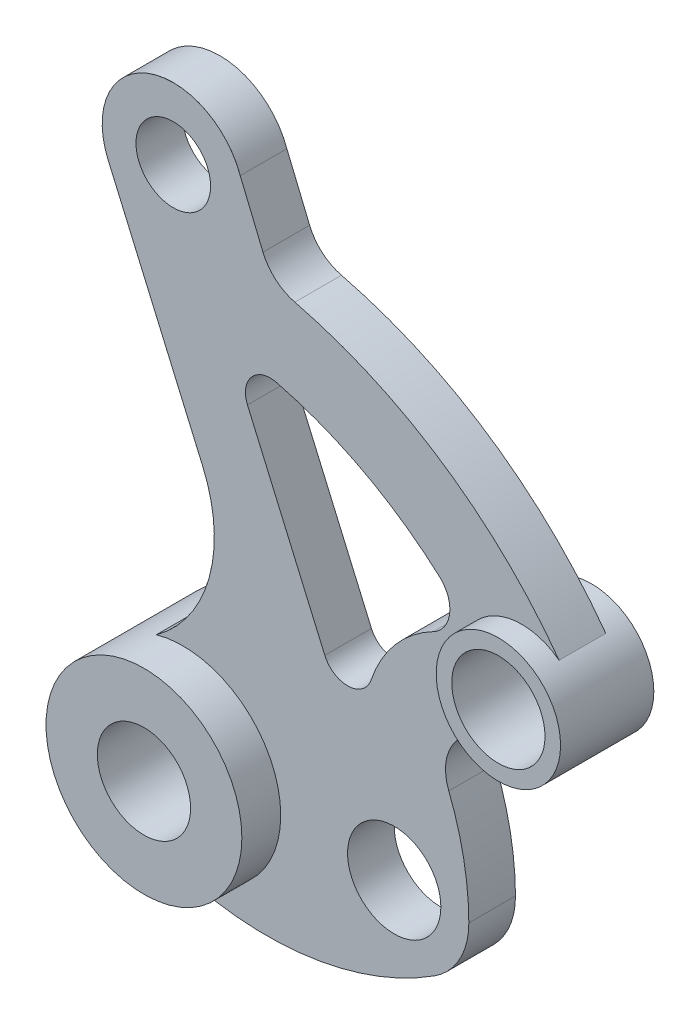
ISO-10303-21;
HEADER;
FILE_DESCRIPTION(('STEP AP214'),'2;1');
FILE_NAME('part.step','',(''),(''),'','','');
FILE_SCHEMA(('AUTOMOTIVE_DESIGN { 1 0 10303 214 1 1 1 1 }'));
ENDSEC;
DATA;
#1=APPLICATION_CONTEXT('core data for automotive mechanical design processes');
#2=APPLICATION_PROTOCOL_DEFINITION('international standard','automotive_design',2000,#1);
#3=PRODUCT_CONTEXT('',#1,'mechanical');
#4=PRODUCT('Part','Part','',(#3));
#5=PRODUCT_RELATED_PRODUCT_CATEGORY('part','',(#4));
#6=PRODUCT_DEFINITION_FORMATION('','',#4);
#7=PRODUCT_DEFINITION_CONTEXT('part definition',#1,'design');
#8=PRODUCT_DEFINITION('design','',#6,#7);
#9=PRODUCT_DEFINITION_SHAPE('','',#8);
#10=(LENGTH_UNIT() NAMED_UNIT(*) SI_UNIT(.MILLI.,.METRE.));
#11=(NAMED_UNIT(*) PLANE_ANGLE_UNIT() SI_UNIT($,.RADIAN.));
#12=(NAMED_UNIT(*) SI_UNIT($,.STERADIAN.) SOLID_ANGLE_UNIT());
#13=UNCERTAINTY_MEASURE_WITH_UNIT(LENGTH_MEASURE(1.E-05),#10,'distance_accuracy_value','');
#14=(GEOMETRIC_REPRESENTATION_CONTEXT(3) GLOBAL_UNCERTAINTY_ASSIGNED_CONTEXT((#13)) GLOBAL_UNIT_ASSIGNED_CONTEXT((#10,
#11,#12)) REPRESENTATION_CONTEXT('',''));
#15=CARTESIAN_POINT('',(0.,0.,0.));
#16=DIRECTION('',(0.,0.,1.));
#17=DIRECTION('',(1.,0.,0.));
#18=AXIS2_PLACEMENT_3D('',#15,#16,#17);
#19=CARTESIAN_POINT('',(0.,0.,15.));
#20=DIRECTION('',(0.,0.,1.));
#21=DIRECTION('',(1.,0.,0.));
#22=AXIS2_PLACEMENT_3D('',#19,#20,#21);
#23=PLANE('',#22);
#24=CARTESIAN_POINT('',(-3.06784573961168,163.971303350671,15.));
#25=DIRECTION('',(0.,0.,1.));
#26=DIRECTION('',(1.,0.,0.));
#27=AXIS2_PLACEMENT_3D('',#24,#25,#26);
#28=CIRCLE('',#27,12.000000000031);
#29=CARTESIAN_POINT('',(8.93215426041928,163.971303350671,15.));
#30=VERTEX_POINT('',#29);
#31=EDGE_CURVE('E225',#30,#30,#28,.T.);
#32=ORIENTED_EDGE('',*,*,#31,.F.);
#33=EDGE_LOOP('',(#32));
#34=FACE_BOUND('',#33,.T.);
#35=CARTESIAN_POINT('',(67.9996451646292,0.219675862409967,15.));
#36=DIRECTION('',(0.,0.,1.));
#37=DIRECTION('',(1.,0.,0.));
#38=AXIS2_PLACEMENT_3D('',#35,#36,#37);
#39=CIRCLE('',#38,14.9999999999901);
#40=CARTESIAN_POINT('',(82.9996451646192,0.219675862409967,15.));
#41=VERTEX_POINT('',#40);
#42=EDGE_CURVE('E222',#41,#41,#39,.T.);
#43=ORIENTED_EDGE('',*,*,#42,.F.);
#44=EDGE_LOOP('',(#43));
#45=FACE_BOUND('',#44,.T.);
#46=DIRECTION('',(0.398118875645799,-0.917333832829971,0.));
#47=VECTOR('',#46,1.);
#48=CARTESIAN_POINT('',(57.3020213071531,24.8688268965916,15.));
#49=LINE('',#48,#47);
#50=CARTESIAN_POINT('',(20.8018674677098,108.971410493279,15.));
#51=VERTEX_POINT('',#50);
#52=CARTESIAN_POINT('',(45.6745977520915,51.6603951145019,15.));
#53=VERTEX_POINT('',#52);
#54=EDGE_CURVE('E460',#51,#53,#49,.T.);
#55=ORIENTED_EDGE('',*,*,#54,.F.);
#56=CARTESIAN_POINT('',(28.1405381303495,112.156361498446,15.));
#57=DIRECTION('',(0.,0.,1.));
#58=DIRECTION('',(1.,0.,0.));
#59=AXIS2_PLACEMENT_3D('',#56,#57,#58);
#60=CIRCLE('',#59,7.99999999999999);
#61=CARTESIAN_POINT('',(30.0874281839262,119.915847249401,15.));
#62=VERTEX_POINT('',#61);
#63=EDGE_CURVE('E453',#51,#62,#60,.F.);
#64=ORIENTED_EDGE('',*,*,#63,.T.);
#65=CARTESIAN_POINT('',(0.,0.,15.));
#66=DIRECTION('',(0.,0.,1.));
#67=DIRECTION('',(1.,0.,0.));
#68=AXIS2_PLACEMENT_3D('',#65,#66,#67);
#69=CIRCLE('',#68,123.632777839312);
#70=CARTESIAN_POINT('',(82.5809627863903,92.0078710846932,15.));
#71=VERTEX_POINT('',#70);
#72=EDGE_CURVE('E455',#71,#62,#69,.T.);
#73=ORIENTED_EDGE('',*,*,#72,.F.);
#74=CARTESIAN_POINT('',(75.9014264830224,84.565842142799,15.));
#75=DIRECTION('',(0.,0.,1.));
#76=DIRECTION('',(1.,0.,0.));
#77=AXIS2_PLACEMENT_3D('',#74,#75,#76);
#78=CIRCLE('',#77,10.);
#79=CARTESIAN_POINT('',(80.5286057442506,75.7007864698515,15.));
#80=VERTEX_POINT('',#79);
#81=EDGE_CURVE('E446',#80,#71,#78,.T.);
#82=ORIENTED_EDGE('',*,*,#81,.F.);
#83=CARTESIAN_POINT('',(99.5000407152862,39.3540582107665,15.));
#84=DIRECTION('',(0.,0.,1.));
#85=DIRECTION('',(1.,0.,0.));
#86=AXIS2_PLACEMENT_3D('',#83,#84,#85);
#87=CIRCLE('',#86,41.);
#88=CARTESIAN_POINT('',(60.6029455250266,52.316156256989,15.));
#89=VERTEX_POINT('',#88);
#90=EDGE_CURVE('E447',#89,#80,#87,.F.);
#91=ORIENTED_EDGE('',*,*,#90,.F.);
#92=CARTESIAN_POINT('',(53.013268414732,54.8453461196665,15.));
#93=DIRECTION('',(0.,0.,1.));
#94=DIRECTION('',(1.,0.,0.));
#95=AXIS2_PLACEMENT_3D('',#92,#93,#94);
#96=CIRCLE('',#95,7.99999999999999);
#97=EDGE_CURVE('E394',#53,#89,#96,.T.);
#98=ORIENTED_EDGE('',*,*,#97,.F.);
#99=EDGE_LOOP('',(#55,#64,#73,#82,#91,#98));
#100=FACE_BOUND('',#99,.T.);
#101=DIRECTION('',(0.383451553640761,-0.923560992035982,0.));
#102=VECTOR('',#101,1.);
#103=CARTESIAN_POINT('',(76.5503269943444,31.7827864870954,15.));
#104=LINE('',#103,#102);
#105=CARTESIAN_POINT('',(18.3868968232772,171.872127002147,15.));
#106=VERTEX_POINT('',#105);
#107=CARTESIAN_POINT('',(25.7921859401268,154.036141991435,15.));
#108=VERTEX_POINT('',#107);
#109=EDGE_CURVE('E403',#106,#108,#104,.T.);
#110=ORIENTED_EDGE('',*,*,#109,.F.);
#111=CARTESIAN_POINT('',(-3.06784573961168,163.971303350671,15.));
#112=DIRECTION('',(0.,0.,1.));
#113=DIRECTION('',(1.,0.,0.));
#114=AXIS2_PLACEMENT_3D('',#111,#112,#113);
#115=CIRCLE('',#114,22.8632673258124);
#116=CARTESIAN_POINT('',(-24.0410943866144,154.869005069327,15.));
#117=VERTEX_POINT('',#116);
#118=EDGE_CURVE('E230',#106,#117,#115,.T.);
#119=ORIENTED_EDGE('',*,*,#118,.T.);
#120=DIRECTION('',(0.398118875645899,-0.917333832829927,0.));
#121=VECTOR('',#120,1.);
#122=CARTESIAN_POINT('',(6.41253141271611,84.6986539832474,15.));
#123=LINE('',#122,#121);
#124=CARTESIAN_POINT('',(6.4125314127161,84.6986539832473,15.));
#125=VERTEX_POINT('',#124);
#126=EDGE_CURVE('E214',#117,#125,#123,.T.);
#127=ORIENTED_EDGE('',*,*,#126,.T.);
#128=CARTESIAN_POINT('',(-34.876664402959,66.7793233904254,15.));
#129=DIRECTION('',(0.,0.,1.));
#130=DIRECTION('',(1.,0.,0.));
#131=AXIS2_PLACEMENT_3D('',#128,#129,#130);
#132=CIRCLE('',#131,45.0100000000001);
#133=CARTESIAN_POINT('',(-8.446752371103,30.346373331607,15.));
#134=VERTEX_POINT('',#133);
#135=EDGE_CURVE('E208',#125,#134,#132,.F.);
#136=ORIENTED_EDGE('',*,*,#135,.T.);
#137=CARTESIAN_POINT('',(0.,0.,15.));
#138=DIRECTION('',(0.,0.,1.));
#139=DIRECTION('',(1.,0.,0.));
#140=AXIS2_PLACEMENT_3D('',#137,#138,#139);
#141=CIRCLE('',#140,31.5);
#142=CARTESIAN_POINT('',(-2.21180302605378,-31.4222521053781,15.));
#143=VERTEX_POINT('',#142);
#144=EDGE_CURVE('E442',#134,#143,#141,.F.);
#145=ORIENTED_EDGE('',*,*,#144,.T.);
#146=CARTESIAN_POINT('',(27.0041064706894,64.2147210393117,15.));
#147=DIRECTION('',(0.,0.,1.));
#148=DIRECTION('',(1.,0.,0.));
#149=AXIS2_PLACEMENT_3D('',#146,#147,#148);
#150=CIRCLE('',#149,100.);
#151=CARTESIAN_POINT('',(80.9456047521891,-19.9892857724011,15.));
#152=VERTEX_POINT('',#151);
#153=EDGE_CURVE('E470',#143,#152,#150,.T.);
#154=ORIENTED_EDGE('',*,*,#153,.T.);
#155=CARTESIAN_POINT('',(67.9996451646292,0.219675862409967,15.));
#156=DIRECTION('',(0.,0.,1.));
#157=DIRECTION('',(1.,0.,0.));
#158=AXIS2_PLACEMENT_3D('',#155,#156,#157);
#159=CIRCLE('',#158,24.);
#160=CARTESIAN_POINT('',(91.999519928616,0.29720851973114,15.));
#161=VERTEX_POINT('',#160);
#162=EDGE_CURVE('E465',#152,#161,#159,.T.);
#163=ORIENTED_EDGE('',*,*,#162,.T.);
#164=CARTESIAN_POINT('',(0.,0.,15.));
#165=DIRECTION('',(0.,0.,1.));
#166=DIRECTION('',(1.,0.,0.));
#167=AXIS2_PLACEMENT_3D('',#164,#165,#166);
#168=CIRCLE('',#167,92.);
#169=CARTESIAN_POINT('',(85.5514368766947,33.8371341625282,15.));
#170=VERTEX_POINT('',#169);
#171=EDGE_CURVE('E464',#161,#170,#168,.T.);
#172=ORIENTED_EDGE('',*,*,#171,.T.);
#173=CARTESIAN_POINT('',(99.5000407152862,39.3540582107665,15.));
#174=DIRECTION('',(0.,0.,1.));
#175=DIRECTION('',(1.,0.,0.));
#176=AXIS2_PLACEMENT_3D('',#173,#174,#175);
#177=CIRCLE('',#176,15.);
#178=CARTESIAN_POINT('',(99.5862507147772,54.3538104699202,15.));
#179=VERTEX_POINT('',#178);
#180=EDGE_CURVE('E200',#170,#179,#177,.F.);
#181=ORIENTED_EDGE('',*,*,#180,.T.);
#182=CARTESIAN_POINT('',(108.999645164629,72.,15.));
#183=DIRECTION('',(0.,0.,1.));
#184=DIRECTION('',(1.,0.,0.));
#185=AXIS2_PLACEMENT_3D('',#182,#183,#184);
#186=CIRCLE('',#185,20.);
#187=CARTESIAN_POINT('',(121.045727624012,87.9653342395873,15.));
#188=VERTEX_POINT('',#187);
#189=EDGE_CURVE('E203',#179,#188,#186,.F.);
#190=ORIENTED_EDGE('',*,*,#189,.T.);
#191=CARTESIAN_POINT('',(0.,0.,15.));
#192=DIRECTION('',(0.,0.,1.));
#193=DIRECTION('',(1.,0.,0.));
#194=AXIS2_PLACEMENT_3D('',#191,#192,#193);
#195=CIRCLE('',#194,149.632777839312);
#196=CARTESIAN_POINT('',(36.0334160533632,145.229339774834,15.));
#197=VERTEX_POINT('',#196);
#198=EDGE_CURVE('E184',#188,#197,#195,.T.);
#199=ORIENTED_EDGE('',*,*,#198,.T.);
#200=CARTESIAN_POINT('',(39.6456008206666,159.787915296047,15.));
#201=DIRECTION('',(0.,0.,1.));
#202=DIRECTION('',(1.,0.,0.));
#203=AXIS2_PLACEMENT_3D('',#200,#201,#202);
#204=CIRCLE('',#203,15.);
#205=EDGE_CURVE('E197',#108,#197,#204,.T.);
#206=ORIENTED_EDGE('',*,*,#205,.F.);
#207=EDGE_LOOP('',(#110,#119,#127,#136,#145,#154,#163,#172,#181,#190,#199,#206));
#208=FACE_BOUND('',#207,.T.);
#209=ADVANCED_FACE('F50',(#34,#45,#100,#208),#23,.T.);
#210=CARTESIAN_POINT('',(0.,0.,0.));
#211=DIRECTION('',(0.,0.,1.));
#212=DIRECTION('',(1.,0.,0.));
#213=AXIS2_PLACEMENT_3D('',#210,#211,#212);
#214=PLANE('',#213);
#215=CARTESIAN_POINT('',(-3.06784573961168,163.971303350671,0.));
#216=DIRECTION('',(0.,0.,1.));
#217=DIRECTION('',(1.,0.,0.));
#218=AXIS2_PLACEMENT_3D('',#215,#216,#217);
#219=CIRCLE('',#218,12.000000000031);
#220=CARTESIAN_POINT('',(8.93215426041928,163.971303350671,0.));
#221=VERTEX_POINT('',#220);
#222=EDGE_CURVE('E221',#221,#221,#219,.T.);
#223=ORIENTED_EDGE('',*,*,#222,.T.);
#224=EDGE_LOOP('',(#223));
#225=FACE_BOUND('',#224,.T.);
#226=CARTESIAN_POINT('',(67.9996451646292,0.219675862409967,0.));
#227=DIRECTION('',(0.,0.,1.));
#228=DIRECTION('',(1.,0.,0.));
#229=AXIS2_PLACEMENT_3D('',#226,#227,#228);
#230=CIRCLE('',#229,14.9999999999901);
#231=CARTESIAN_POINT('',(82.9996451646192,0.219675862409967,0.));
#232=VERTEX_POINT('',#231);
#233=EDGE_CURVE('E218',#232,#232,#230,.T.);
#234=ORIENTED_EDGE('',*,*,#233,.T.);
#235=EDGE_LOOP('',(#234));
#236=FACE_BOUND('',#235,.T.);
#237=DIRECTION('',(0.398118875645799,-0.917333832829971,0.));
#238=VECTOR('',#237,1.);
#239=CARTESIAN_POINT('',(57.3020213071531,24.8688268965916,0.));
#240=LINE('',#239,#238);
#241=CARTESIAN_POINT('',(20.8018674677098,108.971410493279,0.));
#242=VERTEX_POINT('',#241);
#243=CARTESIAN_POINT('',(45.6745977520915,51.6603951145019,0.));
#244=VERTEX_POINT('',#243);
#245=EDGE_CURVE('E417',#242,#244,#240,.T.);
#246=ORIENTED_EDGE('',*,*,#245,.T.);
#247=CARTESIAN_POINT('',(53.013268414732,54.8453461196665,0.));
#248=DIRECTION('',(0.,0.,1.));
#249=DIRECTION('',(1.,0.,0.));
#250=AXIS2_PLACEMENT_3D('',#247,#248,#249);
#251=CIRCLE('',#250,7.99999999999999);
#252=CARTESIAN_POINT('',(60.6029455250266,52.316156256989,0.));
#253=VERTEX_POINT('',#252);
#254=EDGE_CURVE('E405',#244,#253,#251,.T.);
#255=ORIENTED_EDGE('',*,*,#254,.T.);
#256=CARTESIAN_POINT('',(99.5000407152862,39.3540582107665,0.));
#257=DIRECTION('',(0.,0.,1.));
#258=DIRECTION('',(1.,0.,0.));
#259=AXIS2_PLACEMENT_3D('',#256,#257,#258);
#260=CIRCLE('',#259,41.);
#261=CARTESIAN_POINT('',(80.5286057442506,75.7007864698515,0.));
#262=VERTEX_POINT('',#261);
#263=EDGE_CURVE('E407',#253,#262,#260,.F.);
#264=ORIENTED_EDGE('',*,*,#263,.T.);
#265=CARTESIAN_POINT('',(75.9014264830224,84.565842142799,0.));
#266=DIRECTION('',(0.,0.,1.));
#267=DIRECTION('',(1.,0.,0.));
#268=AXIS2_PLACEMENT_3D('',#265,#266,#267);
#269=CIRCLE('',#268,10.);
#270=CARTESIAN_POINT('',(82.5809627863903,92.0078710846932,0.));
#271=VERTEX_POINT('',#270);
#272=EDGE_CURVE('E406',#262,#271,#269,.T.);
#273=ORIENTED_EDGE('',*,*,#272,.T.);
#274=CARTESIAN_POINT('',(0.,0.,0.));
#275=DIRECTION('',(0.,0.,1.));
#276=DIRECTION('',(1.,0.,0.));
#277=AXIS2_PLACEMENT_3D('',#274,#275,#276);
#278=CIRCLE('',#277,123.632777839312);
#279=CARTESIAN_POINT('',(30.0874281839262,119.915847249401,0.));
#280=VERTEX_POINT('',#279);
#281=EDGE_CURVE('E415',#271,#280,#278,.T.);
#282=ORIENTED_EDGE('',*,*,#281,.T.);
#283=CARTESIAN_POINT('',(28.1405381303495,112.156361498446,0.));
#284=DIRECTION('',(0.,0.,1.));
#285=DIRECTION('',(1.,0.,0.));
#286=AXIS2_PLACEMENT_3D('',#283,#284,#285);
#287=CIRCLE('',#286,7.99999999999999);
#288=EDGE_CURVE('E413',#242,#280,#287,.F.);
#289=ORIENTED_EDGE('',*,*,#288,.F.);
#290=EDGE_LOOP('',(#246,#255,#264,#273,#282,#289));
#291=FACE_BOUND('',#290,.T.);
#292=CARTESIAN_POINT('',(108.999645164629,72.,0.));
#293=DIRECTION('',(0.,0.,1.));
#294=DIRECTION('',(1.,0.,0.));
#295=AXIS2_PLACEMENT_3D('',#292,#293,#294);
#296=CIRCLE('',#295,20.);
#297=CARTESIAN_POINT('',(99.5862507147772,54.3538104699202,0.));
#298=VERTEX_POINT('',#297);
#299=CARTESIAN_POINT('',(121.045727624012,87.9653342395873,0.));
#300=VERTEX_POINT('',#299);
#301=EDGE_CURVE('E207',#298,#300,#296,.F.);
#302=ORIENTED_EDGE('',*,*,#301,.F.);
#303=CARTESIAN_POINT('',(99.5000407152862,39.3540582107665,0.));
#304=DIRECTION('',(0.,0.,1.));
#305=DIRECTION('',(1.,0.,0.));
#306=AXIS2_PLACEMENT_3D('',#303,#304,#305);
#307=CIRCLE('',#306,15.);
#308=CARTESIAN_POINT('',(85.5514368766947,33.8371341625282,0.));
#309=VERTEX_POINT('',#308);
#310=EDGE_CURVE('E428',#309,#298,#307,.F.);
#311=ORIENTED_EDGE('',*,*,#310,.F.);
#312=CARTESIAN_POINT('',(0.,0.,0.));
#313=DIRECTION('',(0.,0.,1.));
#314=DIRECTION('',(1.,0.,0.));
#315=AXIS2_PLACEMENT_3D('',#312,#313,#314);
#316=CIRCLE('',#315,92.);
#317=CARTESIAN_POINT('',(91.999519928616,0.29720851973114,0.));
#318=VERTEX_POINT('',#317);
#319=EDGE_CURVE('E429',#318,#309,#316,.T.);
#320=ORIENTED_EDGE('',*,*,#319,.F.);
#321=CARTESIAN_POINT('',(67.9996451646292,0.219675862409967,0.));
#322=DIRECTION('',(0.,0.,1.));
#323=DIRECTION('',(1.,0.,0.));
#324=AXIS2_PLACEMENT_3D('',#321,#322,#323);
#325=CIRCLE('',#324,24.);
#326=CARTESIAN_POINT('',(80.9456047521891,-19.9892857724011,0.));
#327=VERTEX_POINT('',#326);
#328=EDGE_CURVE('E435',#327,#318,#325,.T.);
#329=ORIENTED_EDGE('',*,*,#328,.F.);
#330=CARTESIAN_POINT('',(27.0041064706894,64.2147210393117,0.));
#331=DIRECTION('',(0.,0.,1.));
#332=DIRECTION('',(1.,0.,0.));
#333=AXIS2_PLACEMENT_3D('',#330,#331,#332);
#334=CIRCLE('',#333,100.);
#335=CARTESIAN_POINT('',(-2.21180302605378,-31.4222521053781,0.));
#336=VERTEX_POINT('',#335);
#337=EDGE_CURVE('E434',#336,#327,#334,.T.);
#338=ORIENTED_EDGE('',*,*,#337,.F.);
#339=CARTESIAN_POINT('',(0.,0.,0.));
#340=DIRECTION('',(0.,0.,1.));
#341=DIRECTION('',(1.,0.,0.));
#342=AXIS2_PLACEMENT_3D('',#339,#340,#341);
#343=CIRCLE('',#342,31.5);
#344=CARTESIAN_POINT('',(-8.47443725483162,30.3386537805144,0.));
#345=VERTEX_POINT('',#344);
#346=EDGE_CURVE('E212',#345,#336,#343,.F.);
#347=ORIENTED_EDGE('',*,*,#346,.F.);
#348=CARTESIAN_POINT('',(-34.876664402959,66.7793233904254,0.));
#349=DIRECTION('',(0.,0.,1.));
#350=DIRECTION('',(1.,0.,0.));
#351=AXIS2_PLACEMENT_3D('',#348,#349,#350);
#352=CIRCLE('',#351,45.0000000000001);
#353=CARTESIAN_POINT('',(6.40335807438781,84.6946727944909,0.));
#354=VERTEX_POINT('',#353);
#355=EDGE_CURVE('E440',#354,#345,#352,.F.);
#356=ORIENTED_EDGE('',*,*,#355,.F.);
#357=DIRECTION('',(0.398118875645899,-0.917333832829928,0.));
#358=VECTOR('',#357,1.);
#359=CARTESIAN_POINT('',(36.3195993218346,15.7625474265039,0.));
#360=LINE('',#359,#358);
#361=CARTESIAN_POINT('',(-24.0502677249427,154.865023880571,0.));
#362=VERTEX_POINT('',#361);
#363=EDGE_CURVE('E353',#362,#354,#360,.T.);
#364=ORIENTED_EDGE('',*,*,#363,.F.);
#365=CARTESIAN_POINT('',(-3.06784573961168,163.971303350671,0.));
#366=DIRECTION('',(0.,0.,1.));
#367=DIRECTION('',(1.,0.,0.));
#368=AXIS2_PLACEMENT_3D('',#365,#366,#367);
#369=CIRCLE('',#368,22.8732673258124);
#370=CARTESIAN_POINT('',(18.47121984072,171.669031072814,0.));
#371=VERTEX_POINT('',#370);
#372=EDGE_CURVE('E439',#371,#362,#369,.T.);
#373=ORIENTED_EDGE('',*,*,#372,.F.);
#374=DIRECTION('',(0.383451553640761,-0.923560992035982,0.));
#375=VECTOR('',#374,1.);
#376=CARTESIAN_POINT('',(76.5503269943444,31.7827864870954,0.));
#377=LINE('',#376,#375);
#378=CARTESIAN_POINT('',(25.7921859401268,154.036141991435,0.));
#379=VERTEX_POINT('',#378);
#380=EDGE_CURVE('E376',#371,#379,#377,.T.);
#381=ORIENTED_EDGE('',*,*,#380,.T.);
#382=CARTESIAN_POINT('',(39.6456008206666,159.787915296047,0.));
#383=DIRECTION('',(0.,0.,1.));
#384=DIRECTION('',(1.,0.,0.));
#385=AXIS2_PLACEMENT_3D('',#382,#383,#384);
#386=CIRCLE('',#385,15.);
#387=CARTESIAN_POINT('',(36.0334160533632,145.229339774834,0.));
#388=VERTEX_POINT('',#387);
#389=EDGE_CURVE('E423',#379,#388,#386,.T.);
#390=ORIENTED_EDGE('',*,*,#389,.T.);
#391=CARTESIAN_POINT('',(0.,0.,0.));
#392=DIRECTION('',(0.,0.,1.));
#393=DIRECTION('',(1.,0.,0.));
#394=AXIS2_PLACEMENT_3D('',#391,#392,#393);
#395=CIRCLE('',#394,149.632777839312);
#396=EDGE_CURVE('E425',#300,#388,#395,.T.);
#397=ORIENTED_EDGE('',*,*,#396,.F.);
#398=EDGE_LOOP('',(#302,#311,#320,#329,#338,#347,#356,#364,#373,#381,#390,#397));
#399=FACE_BOUND('',#398,.T.);
#400=ADVANCED_FACE('F277',(#225,#236,#291,#399),#214,.F.);
#401=CARTESIAN_POINT('',(99.5000407152862,39.3540582107665,15.));
#402=DIRECTION('',(0.,0.,-1.));
#403=DIRECTION('',(-1.,0.,0.));
#404=AXIS2_PLACEMENT_3D('',#401,#402,#403);
#405=CYLINDRICAL_SURFACE('',#404,15.);
#406=DIRECTION('',(0.,0.,-1.));
#407=VECTOR('',#406,1.);
#408=CARTESIAN_POINT('',(99.5862507147772,54.3538104699202,7.5));
#409=LINE('',#408,#407);
#410=EDGE_CURVE('E201',#179,#298,#409,.T.);
#411=ORIENTED_EDGE('',*,*,#410,.F.);
#412=ORIENTED_EDGE('',*,*,#180,.F.);
#413=DIRECTION('',(0.,0.,-1.));
#414=VECTOR('',#413,1.);
#415=CARTESIAN_POINT('',(85.5514368766947,33.8371341625282,15.));
#416=LINE('',#415,#414);
#417=EDGE_CURVE('E390',#170,#309,#416,.T.);
#418=ORIENTED_EDGE('',*,*,#417,.T.);
#419=ORIENTED_EDGE('',*,*,#310,.T.);
#420=EDGE_LOOP('',(#411,#412,#418,#419));
#421=FACE_BOUND('',#420,.T.);
#422=ADVANCED_FACE('F281',(#421),#405,.F.);
#423=CARTESIAN_POINT('',(0.,0.,15.));
#424=DIRECTION('',(0.,0.,-1.));
#425=DIRECTION('',(-1.,0.,0.));
#426=AXIS2_PLACEMENT_3D('',#423,#424,#425);
#427=CYLINDRICAL_SURFACE('',#426,149.632777839312);
#428=DIRECTION('',(0.,0.,-1.));
#429=VECTOR('',#428,1.);
#430=CARTESIAN_POINT('',(121.045727624012,87.9653342395873,7.5));
#431=LINE('',#430,#429);
#432=EDGE_CURVE('E186',#300,#188,#431,.F.);
#433=ORIENTED_EDGE('',*,*,#432,.F.);
#434=ORIENTED_EDGE('',*,*,#396,.T.);
#435=DIRECTION('',(0.,0.,-1.));
#436=VECTOR('',#435,1.);
#437=CARTESIAN_POINT('',(36.0334160533632,145.229339774834,15.));
#438=LINE('',#437,#436);
#439=EDGE_CURVE('E195',#197,#388,#438,.T.);
#440=ORIENTED_EDGE('',*,*,#439,.F.);
#441=ORIENTED_EDGE('',*,*,#198,.F.);
#442=EDGE_LOOP('',(#433,#434,#440,#441));
#443=FACE_BOUND('',#442,.T.);
#444=ADVANCED_FACE('F190',(#443),#427,.T.);
#445=CARTESIAN_POINT('',(-34.876664402959,66.7793233904254,15.));
#446=DIRECTION('',(0.,0.,-1.));
#447=DIRECTION('',(-1.,0.,0.));
#448=AXIS2_PLACEMENT_3D('',#445,#446,#447);
#449=CYLINDRICAL_SURFACE('',#448,45.0000000000001);
#450=DIRECTION('',(0.,0.,-1.));
#451=VECTOR('',#450,1.);
#452=CARTESIAN_POINT('',(-8.47443725483162,30.3386537805144,7.5));
#453=LINE('',#452,#451);
#454=CARTESIAN_POINT('',(-8.47443725483162,30.3386537805144,14.99));
#455=VERTEX_POINT('',#454);
#456=EDGE_CURVE('E472',#455,#345,#453,.T.);
#457=ORIENTED_EDGE('',*,*,#456,.F.);
#458=CARTESIAN_POINT('',(-34.876664402959,66.7793233904254,14.99));
#459=DIRECTION('',(0.,0.,1.));
#460=DIRECTION('',(1.,0.,0.));
#461=AXIS2_PLACEMENT_3D('',#458,#459,#460);
#462=CIRCLE('',#461,45.0000000000001);
#463=CARTESIAN_POINT('',(6.40335807438781,84.6946727944909,14.99));
#464=VERTEX_POINT('',#463);
#465=EDGE_CURVE('E68',#455,#464,#462,.T.);
#466=ORIENTED_EDGE('',*,*,#465,.T.);
#467=DIRECTION('',(0.,0.,-1.));
#468=VECTOR('',#467,1.);
#469=CARTESIAN_POINT('',(6.40335807438781,84.6946727944909,15.));
#470=LINE('',#469,#468);
#471=EDGE_CURVE('E347',#464,#354,#470,.T.);
#472=ORIENTED_EDGE('',*,*,#471,.T.);
#473=ORIENTED_EDGE('',*,*,#355,.T.);
#474=EDGE_LOOP('',(#457,#466,#472,#473));
#475=FACE_BOUND('',#474,.T.);
#476=ADVANCED_FACE('F321',(#475),#449,.F.);
#477=CARTESIAN_POINT('',(27.0041064706894,64.2147210393117,15.));
#478=DIRECTION('',(0.,0.,-1.));
#479=DIRECTION('',(-1.,0.,0.));
#480=AXIS2_PLACEMENT_3D('',#477,#478,#479);
#481=CYLINDRICAL_SURFACE('',#480,100.);
#482=DIRECTION('',(0.,0.,-1.));
#483=VECTOR('',#482,1.);
#484=CARTESIAN_POINT('',(-2.21180302605377,-31.4222521053781,7.5));
#485=LINE('',#484,#483);
#486=EDGE_CURVE('E474',#336,#143,#485,.F.);
#487=ORIENTED_EDGE('',*,*,#486,.F.);
#488=ORIENTED_EDGE('',*,*,#337,.T.);
#489=DIRECTION('',(0.,0.,-1.));
#490=VECTOR('',#489,1.);
#491=CARTESIAN_POINT('',(80.9456047521891,-19.9892857724011,15.));
#492=LINE('',#491,#490);
#493=EDGE_CURVE('E351',#152,#327,#492,.T.);
#494=ORIENTED_EDGE('',*,*,#493,.F.);
#495=ORIENTED_EDGE('',*,*,#153,.F.);
#496=EDGE_LOOP('',(#487,#488,#494,#495));
#497=FACE_BOUND('',#496,.T.);
#498=ADVANCED_FACE('F317',(#497),#481,.T.);
#499=CARTESIAN_POINT('',(57.3020213071531,24.8688268965916,15.));
#500=DIRECTION('',(0.917333832829971,0.398118875645799,0.));
#501=DIRECTION('',(-0.398118875645799,0.917333832829971,0.));
#502=AXIS2_PLACEMENT_3D('',#499,#500,#501);
#503=PLANE('',#502);
#504=ORIENTED_EDGE('',*,*,#245,.F.);
#505=DIRECTION('',(0.,0.,-1.));
#506=VECTOR('',#505,1.);
#507=CARTESIAN_POINT('',(20.8018674677098,108.971410493279,15.));
#508=LINE('',#507,#506);
#509=EDGE_CURVE('E217',#51,#242,#508,.T.);
#510=ORIENTED_EDGE('',*,*,#509,.F.);
#511=ORIENTED_EDGE('',*,*,#54,.T.);
#512=DIRECTION('',(0.,0.,-1.));
#513=VECTOR('',#512,1.);
#514=CARTESIAN_POINT('',(45.6745977520915,51.6603951145019,15.));
#515=LINE('',#514,#513);
#516=EDGE_CURVE('E380',#53,#244,#515,.T.);
#517=ORIENTED_EDGE('',*,*,#516,.T.);
#518=EDGE_LOOP('',(#504,#510,#511,#517));
#519=FACE_BOUND('',#518,.T.);
#520=ADVANCED_FACE('F315',(#519),#503,.T.);
#521=CARTESIAN_POINT('',(28.1405381303495,112.156361498446,15.));
#522=DIRECTION('',(0.,0.,-1.));
#523=DIRECTION('',(-1.,0.,0.));
#524=AXIS2_PLACEMENT_3D('',#521,#522,#523);
#525=CYLINDRICAL_SURFACE('',#524,7.99999999999999);
#526=ORIENTED_EDGE('',*,*,#288,.T.);
#527=DIRECTION('',(0.,0.,-1.));
#528=VECTOR('',#527,1.);
#529=CARTESIAN_POINT('',(30.0874281839262,119.915847249401,15.));
#530=LINE('',#529,#528);
#531=EDGE_CURVE('E393',#62,#280,#530,.T.);
#532=ORIENTED_EDGE('',*,*,#531,.F.);
#533=ORIENTED_EDGE('',*,*,#63,.F.);
#534=ORIENTED_EDGE('',*,*,#509,.T.);
#535=EDGE_LOOP('',(#526,#532,#533,#534));
#536=FACE_BOUND('',#535,.T.);
#537=ADVANCED_FACE('F308',(#536),#525,.F.);
#538=CARTESIAN_POINT('',(0.,0.,15.));
#539=DIRECTION('',(0.,0.,-1.));
#540=DIRECTION('',(-1.,0.,0.));
#541=AXIS2_PLACEMENT_3D('',#538,#539,#540);
#542=CYLINDRICAL_SURFACE('',#541,123.632777839312);
#543=ORIENTED_EDGE('',*,*,#281,.F.);
#544=DIRECTION('',(0.,0.,-1.));
#545=VECTOR('',#544,1.);
#546=CARTESIAN_POINT('',(82.5809627863903,92.0078710846932,15.));
#547=LINE('',#546,#545);
#548=EDGE_CURVE('E399',#71,#271,#547,.T.);
#549=ORIENTED_EDGE('',*,*,#548,.F.);
#550=ORIENTED_EDGE('',*,*,#72,.T.);
#551=ORIENTED_EDGE('',*,*,#531,.T.);
#552=EDGE_LOOP('',(#543,#549,#550,#551));
#553=FACE_BOUND('',#552,.T.);
#554=ADVANCED_FACE('F302',(#553),#542,.F.);
#555=CARTESIAN_POINT('',(75.9014264830224,84.565842142799,15.));
#556=DIRECTION('',(0.,0.,-1.));
#557=DIRECTION('',(-1.,0.,0.));
#558=AXIS2_PLACEMENT_3D('',#555,#556,#557);
#559=CYLINDRICAL_SURFACE('',#558,10.);
#560=ORIENTED_EDGE('',*,*,#272,.F.);
#561=DIRECTION('',(0.,0.,-1.));
#562=VECTOR('',#561,1.);
#563=CARTESIAN_POINT('',(80.5286057442506,75.7007864698515,15.));
#564=LINE('',#563,#562);
#565=EDGE_CURVE('E400',#80,#262,#564,.T.);
#566=ORIENTED_EDGE('',*,*,#565,.F.);
#567=ORIENTED_EDGE('',*,*,#81,.T.);
#568=ORIENTED_EDGE('',*,*,#548,.T.);
#569=EDGE_LOOP('',(#560,#566,#567,#568));
#570=FACE_BOUND('',#569,.T.);
#571=ADVANCED_FACE('F297',(#570),#559,.F.);
#572=CARTESIAN_POINT('',(99.5000407152862,39.3540582107665,15.));
#573=DIRECTION('',(0.,0.,-1.));
#574=DIRECTION('',(-1.,0.,0.));
#575=AXIS2_PLACEMENT_3D('',#572,#573,#574);
#576=CYLINDRICAL_SURFACE('',#575,41.);
#577=ORIENTED_EDGE('',*,*,#263,.F.);
#578=DIRECTION('',(0.,0.,-1.));
#579=VECTOR('',#578,1.);
#580=CARTESIAN_POINT('',(60.6029455250266,52.316156256989,15.));
#581=LINE('',#580,#579);
#582=EDGE_CURVE('E377',#89,#253,#581,.T.);
#583=ORIENTED_EDGE('',*,*,#582,.F.);
#584=ORIENTED_EDGE('',*,*,#90,.T.);
#585=ORIENTED_EDGE('',*,*,#565,.T.);
#586=EDGE_LOOP('',(#577,#583,#584,#585));
#587=FACE_BOUND('',#586,.T.);
#588=ADVANCED_FACE('F260',(#587),#576,.T.);
#589=CARTESIAN_POINT('',(76.5503269943444,31.7827864870954,15.));
#590=DIRECTION('',(0.923560992035982,0.383451553640761,0.));
#591=DIRECTION('',(-0.383451553640761,0.923560992035982,0.));
#592=AXIS2_PLACEMENT_3D('',#589,#590,#591);
#593=PLANE('',#592);
#594=ORIENTED_EDGE('',*,*,#380,.F.);
#595=DIRECTION('',(0.,0.,-1.));
#596=VECTOR('',#595,1.);
#597=CARTESIAN_POINT('',(18.47121984072,171.669031072814,15.));
#598=LINE('',#597,#596);
#599=CARTESIAN_POINT('',(18.47121984072,171.669031072814,14.99));
#600=VERTEX_POINT('',#599);
#601=EDGE_CURVE('E371',#600,#371,#598,.T.);
#602=ORIENTED_EDGE('',*,*,#601,.F.);
#603=CARTESIAN_POINT('',(18.47121984072,171.669031072814,14.99));
#604=CARTESIAN_POINT('',(18.4712198799691,171.669030978281,14.9900320281445));
#605=CARTESIAN_POINT('',(18.471218668792,171.669033895458,14.9900639098042));
#606=CARTESIAN_POINT('',(18.4712141220268,171.669044846554,14.9901261822175));
#607=CARTESIAN_POINT('',(18.4712108165983,171.669052807833,14.9901565876447));
#608=CARTESIAN_POINT('',(18.4712011503697,171.669076089397,14.990224741357));
#609=CARTESIAN_POINT('',(18.4711941623775,171.669092920303,14.9902618701657));
#610=CARTESIAN_POINT('',(18.471178029761,171.669131776464,14.9903329636291));
#611=CARTESIAN_POINT('',(18.4711688717778,171.669153833894,14.990366906789));
#612=CARTESIAN_POINT('',(18.4711407254975,171.669221625526,14.9904593071945));
#613=CARTESIAN_POINT('',(18.4711199948127,171.66927155635,14.9905140963616));
#614=CARTESIAN_POINT('',(18.4710759577119,171.669377621765,14.9906159193656));
#615=CARTESIAN_POINT('',(18.4710526449929,171.669433771539,14.9906629334938));
#616=CARTESIAN_POINT('',(18.4709261415829,171.669738460915,14.9908979573101));
#617=CARTESIAN_POINT('',(18.4708117197002,171.670014051369,14.9910427250163));
#618=CARTESIAN_POINT('',(18.4705775895628,171.67057796475,14.9912994829237));
#619=CARTESIAN_POINT('',(18.4704578385907,171.670866390564,14.9914111151631));
#620=CARTESIAN_POINT('',(18.4693927606332,171.673431680613,14.992338254788));
#621=CARTESIAN_POINT('',(18.468401124195,171.67582008333,14.9927475035864));
#622=CARTESIAN_POINT('',(18.4634596062948,171.687721960193,14.9945765942579));
#623=CARTESIAN_POINT('',(18.459507429588,171.697240962542,14.9953702523444));
#624=CARTESIAN_POINT('',(18.4476356011147,171.725834816389,14.9973309279915));
#625=CARTESIAN_POINT('',(18.4396954926941,171.744958938694,14.9980792382594));
#626=CARTESIAN_POINT('',(18.4238263985654,171.78318039373,14.9991740063444));
#627=CARTESIAN_POINT('',(18.4158974090017,171.802277735749,14.9995207169258));
#628=CARTESIAN_POINT('',(18.4044554141376,171.829836315254,14.9998250965582));
#629=CARTESIAN_POINT('',(18.4009441023856,171.838293473751,14.9998918960054));
#630=CARTESIAN_POINT('',(18.3939206928649,171.855209683903,14.9999790806992));
#631=CARTESIAN_POINT('',(18.390408595079,171.863668735599,14.9999994567031));
#632=CARTESIAN_POINT('',(18.3868968232772,171.872127002147,15.));
#633=B_SPLINE_CURVE_WITH_KNOTS('',3,(#603,#604,#605,#606,#607,#608,#609,#610,#611,#612,#613,
#614,#615,#616,#617,#618,#619,#620,#621,#622,#623,#624,#625,#626,#627,#628,#629,#630,#631,#632),
.UNSPECIFIED.,.F.,.F.,(4,2,2,2,2,2,2,2,2,2,2,2,2,2,4),(0.,9.56935455833691E-05,
0.000190039378958791,0.000313416332849837,0.000437573512543225,0.000667193618088567,
0.000897387139829602,0.001882492500632,0.00287788197187634,0.0106792962262812,
0.0417477971954261,0.103844037896192,0.165901174336529,0.19337232610017,0.220848946845626),.UNSPECIFIED.);
#634=EDGE_CURVE('E60',#600,#106,#633,.T.);
#635=ORIENTED_EDGE('',*,*,#634,.T.);
#636=ORIENTED_EDGE('',*,*,#109,.T.);
#637=DIRECTION('',(0.,0.,-1.));
#638=VECTOR('',#637,1.);
#639=CARTESIAN_POINT('',(25.7921859401268,154.036141991435,15.));
#640=LINE('',#639,#638);
#641=EDGE_CURVE('E392',#108,#379,#640,.T.);
#642=ORIENTED_EDGE('',*,*,#641,.T.);
#643=EDGE_LOOP('',(#594,#602,#635,#636,#642));
#644=FACE_BOUND('',#643,.T.);
#645=ADVANCED_FACE('F255',(#644),#593,.T.);
#646=CARTESIAN_POINT('',(-3.06784573961168,163.971303350671,15.));
#647=DIRECTION('',(0.,0.,-1.));
#648=DIRECTION('',(-1.,0.,0.));
#649=AXIS2_PLACEMENT_3D('',#646,#647,#648);
#650=CYLINDRICAL_SURFACE('',#649,22.8732673258124);
#651=DIRECTION('',(0.,0.,-1.));
#652=VECTOR('',#651,1.);
#653=CARTESIAN_POINT('',(-24.0502677249427,154.865023880571,15.));
#654=LINE('',#653,#652);
#655=CARTESIAN_POINT('',(-24.0502677249427,154.865023880571,14.99));
#656=VERTEX_POINT('',#655);
#657=EDGE_CURVE('E355',#656,#362,#654,.T.);
#658=ORIENTED_EDGE('',*,*,#657,.F.);
#659=CARTESIAN_POINT('',(-3.06784573961168,163.971303350671,14.99));
#660=DIRECTION('',(0.,0.,1.));
#661=DIRECTION('',(1.,0.,0.));
#662=AXIS2_PLACEMENT_3D('',#659,#660,#661);
#663=CIRCLE('',#662,22.8732673258124);
#664=EDGE_CURVE('E235',#656,#600,#663,.F.);
#665=ORIENTED_EDGE('',*,*,#664,.T.);
#666=ORIENTED_EDGE('',*,*,#601,.T.);
#667=ORIENTED_EDGE('',*,*,#372,.T.);
#668=EDGE_LOOP('',(#658,#665,#666,#667));
#669=FACE_BOUND('',#668,.T.);
#670=ADVANCED_FACE('F257',(#669),#650,.T.);
#671=CARTESIAN_POINT('',(36.3195993218346,15.7625474265039,15.));
#672=DIRECTION('',(0.917333832829927,0.398118875645899,0.));
#673=DIRECTION('',(-0.398118875645899,0.917333832829927,0.));
#674=AXIS2_PLACEMENT_3D('',#671,#672,#673);
#675=PLANE('',#674);
#676=ORIENTED_EDGE('',*,*,#471,.F.);
#677=DIRECTION('',(0.398118875645899,-0.917333832829927,0.));
#678=VECTOR('',#677,1.);
#679=CARTESIAN_POINT('',(-24.0502677249427,154.865023880571,14.99));
#680=LINE('',#679,#678);
#681=EDGE_CURVE('E234',#464,#656,#680,.F.);
#682=ORIENTED_EDGE('',*,*,#681,.T.);
#683=ORIENTED_EDGE('',*,*,#657,.T.);
#684=ORIENTED_EDGE('',*,*,#363,.T.);
#685=EDGE_LOOP('',(#676,#682,#683,#684));
#686=FACE_BOUND('',#685,.T.);
#687=ADVANCED_FACE('F335',(#686),#675,.F.);
#688=CARTESIAN_POINT('',(67.9996451646292,0.219675862409967,15.));
#689=DIRECTION('',(0.,0.,-1.));
#690=DIRECTION('',(-1.,0.,0.));
#691=AXIS2_PLACEMENT_3D('',#688,#689,#690);
#692=CYLINDRICAL_SURFACE('',#691,24.);
#693=ORIENTED_EDGE('',*,*,#328,.T.);
#694=DIRECTION('',(0.,0.,-1.));
#695=VECTOR('',#694,1.);
#696=CARTESIAN_POINT('',(91.999519928616,0.29720851973114,15.));
#697=LINE('',#696,#695);
#698=EDGE_CURVE('E381',#161,#318,#697,.T.);
#699=ORIENTED_EDGE('',*,*,#698,.F.);
#700=ORIENTED_EDGE('',*,*,#162,.F.);
#701=ORIENTED_EDGE('',*,*,#493,.T.);
#702=EDGE_LOOP('',(#693,#699,#700,#701));
#703=FACE_BOUND('',#702,.T.);
#704=ADVANCED_FACE('F328',(#703),#692,.T.);
#705=CARTESIAN_POINT('',(0.,0.,15.));
#706=DIRECTION('',(0.,0.,-1.));
#707=DIRECTION('',(-1.,0.,0.));
#708=AXIS2_PLACEMENT_3D('',#705,#706,#707);
#709=CYLINDRICAL_SURFACE('',#708,92.);
#710=ORIENTED_EDGE('',*,*,#319,.T.);
#711=ORIENTED_EDGE('',*,*,#417,.F.);
#712=ORIENTED_EDGE('',*,*,#171,.F.);
#713=ORIENTED_EDGE('',*,*,#698,.T.);
#714=EDGE_LOOP('',(#710,#711,#712,#713));
#715=FACE_BOUND('',#714,.T.);
#716=ADVANCED_FACE('F318',(#715),#709,.T.);
#717=CARTESIAN_POINT('',(39.6456008206666,159.787915296047,15.));
#718=DIRECTION('',(0.,0.,-1.));
#719=DIRECTION('',(-1.,0.,0.));
#720=AXIS2_PLACEMENT_3D('',#717,#718,#719);
#721=CYLINDRICAL_SURFACE('',#720,15.);
#722=ORIENTED_EDGE('',*,*,#389,.F.);
#723=ORIENTED_EDGE('',*,*,#641,.F.);
#724=ORIENTED_EDGE('',*,*,#205,.T.);
#725=ORIENTED_EDGE('',*,*,#439,.T.);
#726=EDGE_LOOP('',(#722,#723,#724,#725));
#727=FACE_BOUND('',#726,.T.);
#728=ADVANCED_FACE('F298',(#727),#721,.F.);
#729=CARTESIAN_POINT('',(53.013268414732,54.8453461196665,15.));
#730=DIRECTION('',(0.,0.,-1.));
#731=DIRECTION('',(-1.,0.,0.));
#732=AXIS2_PLACEMENT_3D('',#729,#730,#731);
#733=CYLINDRICAL_SURFACE('',#732,7.99999999999999);
#734=ORIENTED_EDGE('',*,*,#254,.F.);
#735=ORIENTED_EDGE('',*,*,#516,.F.);
#736=ORIENTED_EDGE('',*,*,#97,.T.);
#737=ORIENTED_EDGE('',*,*,#582,.T.);
#738=EDGE_LOOP('',(#734,#735,#736,#737));
#739=FACE_BOUND('',#738,.T.);
#740=ADVANCED_FACE('F292',(#739),#733,.F.);
#741=CARTESIAN_POINT('',(0.,0.,27.5));
#742=DIRECTION('',(0.,0.,1.));
#743=DIRECTION('',(1.,0.,0.));
#744=AXIS2_PLACEMENT_3D('',#741,#742,#743);
#745=PLANE('',#744);
#746=CARTESIAN_POINT('',(0.,0.,27.5));
#747=DIRECTION('',(0.,0.,1.));
#748=DIRECTION('',(1.,0.,0.));
#749=AXIS2_PLACEMENT_3D('',#746,#747,#748);
#750=CIRCLE('',#749,31.5);
#751=CARTESIAN_POINT('',(31.5,0.,27.5));
#752=VERTEX_POINT('',#751);
#753=EDGE_CURVE('E477',#752,#752,#750,.T.);
#754=ORIENTED_EDGE('',*,*,#753,.T.);
#755=EDGE_LOOP('',(#754));
#756=FACE_BOUND('',#755,.T.);
#757=CARTESIAN_POINT('',(0.,0.,27.5));
#758=DIRECTION('',(0.,0.,1.));
#759=DIRECTION('',(1.,0.,0.));
#760=AXIS2_PLACEMENT_3D('',#757,#758,#759);
#761=CIRCLE('',#760,15.);
#762=CARTESIAN_POINT('',(15.,0.,27.5));
#763=VERTEX_POINT('',#762);
#764=EDGE_CURVE('E478',#763,#763,#761,.T.);
#765=ORIENTED_EDGE('',*,*,#764,.F.);
#766=EDGE_LOOP('',(#765));
#767=FACE_BOUND('',#766,.T.);
#768=ADVANCED_FACE('F294',(#756,#767),#745,.T.);
#769=CARTESIAN_POINT('',(0.,0.,-12.5));
#770=DIRECTION('',(0.,0.,1.));
#771=DIRECTION('',(1.,0.,0.));
#772=AXIS2_PLACEMENT_3D('',#769,#770,#771);
#773=PLANE('',#772);
#774=CARTESIAN_POINT('',(0.,0.,-12.5));
#775=DIRECTION('',(0.,0.,1.));
#776=DIRECTION('',(1.,0.,0.));
#777=AXIS2_PLACEMENT_3D('',#774,#775,#776);
#778=CIRCLE('',#777,31.5);
#779=CARTESIAN_POINT('',(31.5,0.,-12.5));
#780=VERTEX_POINT('',#779);
#781=EDGE_CURVE('E480',#780,#780,#778,.T.);
#782=ORIENTED_EDGE('',*,*,#781,.F.);
#783=EDGE_LOOP('',(#782));
#784=FACE_BOUND('',#783,.T.);
#785=CARTESIAN_POINT('',(0.,0.,-12.5));
#786=DIRECTION('',(0.,0.,1.));
#787=DIRECTION('',(1.,0.,0.));
#788=AXIS2_PLACEMENT_3D('',#785,#786,#787);
#789=CIRCLE('',#788,15.);
#790=CARTESIAN_POINT('',(15.,0.,-12.5));
#791=VERTEX_POINT('',#790);
#792=EDGE_CURVE('E482',#791,#791,#789,.T.);
#793=ORIENTED_EDGE('',*,*,#792,.T.);
#794=EDGE_LOOP('',(#793));
#795=FACE_BOUND('',#794,.T.);
#796=ADVANCED_FACE('F275',(#784,#795),#773,.F.);
#797=CARTESIAN_POINT('',(0.,0.,27.5));
#798=DIRECTION('',(0.,0.,-1.));
#799=DIRECTION('',(-1.,0.,0.));
#800=AXIS2_PLACEMENT_3D('',#797,#798,#799);
#801=CYLINDRICAL_SURFACE('',#800,31.5);
#802=ORIENTED_EDGE('',*,*,#144,.F.);
#803=CARTESIAN_POINT('',(-8.446752371103,30.346373331607,15.));
#804=CARTESIAN_POINT('',(-8.44837142888291,30.3459226740347,15.000000138956));
#805=CARTESIAN_POINT('',(-8.44998739605105,30.3454727391977,14.9999494328257));
#806=CARTESIAN_POINT('',(-8.45322357379161,30.3445714106438,14.999739889843));
#807=CARTESIAN_POINT('',(-8.45484373986164,30.3441200274531,14.9995803283743));
#808=CARTESIAN_POINT('',(-8.45970116156548,30.3427663108703,14.9989285257167));
#809=CARTESIAN_POINT('',(-8.46292768273735,30.3418665420055,14.9982631061361));
#810=CARTESIAN_POINT('',(-8.46658063310479,30.3408472646767,14.996979932819));
#811=CARTESIAN_POINT('',(-8.46713855506633,30.3406915712322,14.9967684533147));
#812=CARTESIAN_POINT('',(-8.46824194317102,30.3403836283711,14.9963080747612));
#813=CARTESIAN_POINT('',(-8.46878737110602,30.3402313895296,14.996059075026));
#814=CARTESIAN_POINT('',(-8.46992695501404,30.3399132789175,14.9954797375469));
#815=CARTESIAN_POINT('',(-8.47051812831081,30.3397482354655,14.9951430165908));
#816=CARTESIAN_POINT('',(-8.47165088852532,30.3394319584449,14.9943897562374));
#817=CARTESIAN_POINT('',(-8.47219271695612,30.3392806576252,14.9939736403283));
#818=CARTESIAN_POINT('',(-8.47288224034075,30.339088097463,14.9933075787244));
#819=CARTESIAN_POINT('',(-8.4730727529685,30.3390348916653,14.9931059076898));
#820=CARTESIAN_POINT('',(-8.47342985191347,30.3389351589448,14.9926799432884));
#821=CARTESIAN_POINT('',(-8.47359640514133,30.3388886412588,14.9924556193502));
#822=CARTESIAN_POINT('',(-8.47389732616603,30.3388045929711,14.9919789025979));
#823=CARTESIAN_POINT('',(-8.47403111981079,30.338767222692,14.9917261089556));
#824=CARTESIAN_POINT('',(-8.47424718022486,30.338706873257,14.9911982317959));
#825=CARTESIAN_POINT('',(-8.47432973862042,30.3386838126518,14.9909232846875));
#826=CARTESIAN_POINT('',(-8.47439885895598,30.3386645055389,14.9905367194068));
#827=CARTESIAN_POINT('',(-8.47441318163701,30.3386605048251,14.9904301076109));
#828=CARTESIAN_POINT('',(-8.47443239979646,30.3386551366626,14.9902156926415));
#829=CARTESIAN_POINT('',(-8.47443727041875,30.338653776157,14.9901078870746));
#830=CARTESIAN_POINT('',(-8.4744372548316,30.3386537805144,14.99));
#831=B_SPLINE_CURVE_WITH_KNOTS('',3,(#803,#804,#805,#806,#807,#808,#809,#810,#811,#812,#813,
#814,#815,#816,#817,#818,#819,#820,#821,#822,#823,#824,#825,#826,#827,#828,#829,#830),
.UNSPECIFIED.,.F.,.F.,(4,2,2,2,2,2,2,2,2,2,2,2,2,4),(0.,0.00503447791115039,0.0101028000611399,
0.0202632435933284,0.0221122814979075,0.0239663727209909,0.0260634672000486,0.0281496737211416,
0.0289956628282193,0.0298428093052719,0.0307038830651737,0.0315600096078799,0.0318825527708133,
0.0322059429838221),.UNSPECIFIED.);
#832=EDGE_CURVE('E11',#134,#455,#831,.T.);
#833=ORIENTED_EDGE('',*,*,#832,.T.);
#834=ORIENTED_EDGE('',*,*,#456,.T.);
#835=ORIENTED_EDGE('',*,*,#346,.T.);
#836=ORIENTED_EDGE('',*,*,#486,.T.);
#837=EDGE_LOOP('',(#802,#833,#834,#835,#836));
#838=FACE_BOUND('',#837,.T.);
#839=ORIENTED_EDGE('',*,*,#753,.F.);
#840=EDGE_LOOP('',(#839));
#841=FACE_BOUND('',#840,.T.);
#842=ORIENTED_EDGE('',*,*,#781,.T.);
#843=EDGE_LOOP('',(#842));
#844=FACE_BOUND('',#843,.T.);
#845=ADVANCED_FACE('F265',(#838,#841,#844),#801,.T.);
#846=CARTESIAN_POINT('',(0.,0.,15.));
#847=DIRECTION('',(0.,0.,-1.));
#848=DIRECTION('',(-1.,0.,0.));
#849=AXIS2_PLACEMENT_3D('',#846,#847,#848);
#850=CYLINDRICAL_SURFACE('',#849,15.);
#851=ORIENTED_EDGE('',*,*,#792,.F.);
#852=EDGE_LOOP('',(#851));
#853=FACE_BOUND('',#852,.T.);
#854=ORIENTED_EDGE('',*,*,#764,.T.);
#855=EDGE_LOOP('',(#854));
#856=FACE_BOUND('',#855,.T.);
#857=ADVANCED_FACE('F258',(#853,#856),#850,.F.);
#858=CARTESIAN_POINT('',(108.999645164629,72.,22.5));
#859=DIRECTION('',(0.,0.,-1.));
#860=DIRECTION('',(-1.,0.,0.));
#861=AXIS2_PLACEMENT_3D('',#858,#859,#860);
#862=CYLINDRICAL_SURFACE('',#861,20.);
#863=CARTESIAN_POINT('',(108.999645164629,72.,22.5));
#864=DIRECTION('',(0.,0.,1.));
#865=DIRECTION('',(1.,0.,0.));
#866=AXIS2_PLACEMENT_3D('',#863,#864,#865);
#867=CIRCLE('',#866,20.);
#868=CARTESIAN_POINT('',(128.999645164629,72.,22.5));
#869=VERTEX_POINT('',#868);
#870=EDGE_CURVE('E489',#869,#869,#867,.T.);
#871=ORIENTED_EDGE('',*,*,#870,.F.);
#872=EDGE_LOOP('',(#871));
#873=FACE_BOUND('',#872,.T.);
#874=CARTESIAN_POINT('',(108.999645164629,72.,-7.5));
#875=DIRECTION('',(0.,0.,1.));
#876=DIRECTION('',(1.,0.,0.));
#877=AXIS2_PLACEMENT_3D('',#874,#875,#876);
#878=CIRCLE('',#877,20.);
#879=CARTESIAN_POINT('',(128.999645164629,72.,-7.5));
#880=VERTEX_POINT('',#879);
#881=EDGE_CURVE('E493',#880,#880,#878,.T.);
#882=ORIENTED_EDGE('',*,*,#881,.T.);
#883=EDGE_LOOP('',(#882));
#884=FACE_BOUND('',#883,.T.);
#885=ORIENTED_EDGE('',*,*,#189,.F.);
#886=ORIENTED_EDGE('',*,*,#410,.T.);
#887=ORIENTED_EDGE('',*,*,#301,.T.);
#888=ORIENTED_EDGE('',*,*,#432,.T.);
#889=EDGE_LOOP('',(#885,#886,#887,#888));
#890=FACE_BOUND('',#889,.T.);
#891=ADVANCED_FACE('F209',(#873,#884,#890),#862,.T.);
#892=CARTESIAN_POINT('',(108.999645164629,72.,22.5));
#893=DIRECTION('',(0.,0.,1.));
#894=DIRECTION('',(1.,0.,0.));
#895=AXIS2_PLACEMENT_3D('',#892,#893,#894);
#896=PLANE('',#895);
#897=ORIENTED_EDGE('',*,*,#870,.T.);
#898=EDGE_LOOP('',(#897));
#899=FACE_BOUND('',#898,.T.);
#900=CARTESIAN_POINT('',(108.999645164629,72.,22.5));
#901=DIRECTION('',(0.,0.,1.));
#902=DIRECTION('',(1.,0.,0.));
#903=AXIS2_PLACEMENT_3D('',#900,#901,#902);
#904=CIRCLE('',#903,15.);
#905=CARTESIAN_POINT('',(123.999645164629,72.,22.5));
#906=VERTEX_POINT('',#905);
#907=EDGE_CURVE('E494',#906,#906,#904,.T.);
#908=ORIENTED_EDGE('',*,*,#907,.F.);
#909=EDGE_LOOP('',(#908));
#910=FACE_BOUND('',#909,.T.);
#911=ADVANCED_FACE('F267',(#899,#910),#896,.T.);
#912=CARTESIAN_POINT('',(108.999645164629,72.,-7.5));
#913=DIRECTION('',(0.,0.,1.));
#914=DIRECTION('',(1.,0.,0.));
#915=AXIS2_PLACEMENT_3D('',#912,#913,#914);
#916=PLANE('',#915);
#917=ORIENTED_EDGE('',*,*,#881,.F.);
#918=EDGE_LOOP('',(#917));
#919=FACE_BOUND('',#918,.T.);
#920=CARTESIAN_POINT('',(108.999645164629,72.,-7.5));
#921=DIRECTION('',(0.,0.,1.));
#922=DIRECTION('',(1.,0.,0.));
#923=AXIS2_PLACEMENT_3D('',#920,#921,#922);
#924=CIRCLE('',#923,15.);
#925=CARTESIAN_POINT('',(123.999645164629,72.,-7.5));
#926=VERTEX_POINT('',#925);
#927=EDGE_CURVE('E500',#926,#926,#924,.T.);
#928=ORIENTED_EDGE('',*,*,#927,.T.);
#929=EDGE_LOOP('',(#928));
#930=FACE_BOUND('',#929,.T.);
#931=ADVANCED_FACE('F544',(#919,#930),#916,.F.);
#932=CARTESIAN_POINT('',(108.999645164629,72.,-12.5));
#933=DIRECTION('',(0.,0.,1.));
#934=DIRECTION('',(1.,0.,0.));
#935=AXIS2_PLACEMENT_3D('',#932,#933,#934);
#936=CYLINDRICAL_SURFACE('',#935,15.);
#937=ORIENTED_EDGE('',*,*,#927,.F.);
#938=EDGE_LOOP('',(#937));
#939=FACE_BOUND('',#938,.T.);
#940=ORIENTED_EDGE('',*,*,#907,.T.);
#941=EDGE_LOOP('',(#940));
#942=FACE_BOUND('',#941,.T.);
#943=ADVANCED_FACE('F545',(#939,#942),#936,.F.);
#944=CARTESIAN_POINT('',(67.9996451646292,0.219675862409967,-7.5));
#945=DIRECTION('',(0.,0.,1.));
#946=DIRECTION('',(1.,0.,0.));
#947=AXIS2_PLACEMENT_3D('',#944,#945,#946);
#948=CYLINDRICAL_SURFACE('',#947,14.9999999999901);
#949=ORIENTED_EDGE('',*,*,#42,.T.);
#950=EDGE_LOOP('',(#949));
#951=FACE_BOUND('',#950,.T.);
#952=ORIENTED_EDGE('',*,*,#233,.F.);
#953=EDGE_LOOP('',(#952));
#954=FACE_BOUND('',#953,.T.);
#955=ADVANCED_FACE('F508',(#951,#954),#948,.F.);
#956=CARTESIAN_POINT('',(-3.06784573961168,163.971303350671,-7.5));
#957=DIRECTION('',(0.,0.,1.));
#958=DIRECTION('',(1.,0.,0.));
#959=AXIS2_PLACEMENT_3D('',#956,#957,#958);
#960=CYLINDRICAL_SURFACE('',#959,12.000000000031);
#961=ORIENTED_EDGE('',*,*,#31,.T.);
#962=EDGE_LOOP('',(#961));
#963=FACE_BOUND('',#962,.T.);
#964=ORIENTED_EDGE('',*,*,#222,.F.);
#965=EDGE_LOOP('',(#964));
#966=FACE_BOUND('',#965,.T.);
#967=ADVANCED_FACE('F506',(#963,#966),#960,.F.);
#968=CARTESIAN_POINT('',(-34.876664402959,66.7793233904254,14.99));
#969=DIRECTION('',(0.,0.,1.));
#970=DIRECTION('',(1.,0.,0.));
#971=AXIS2_PLACEMENT_3D('',#968,#969,#970);
#972=TOROIDAL_SURFACE('',#971,45.0100000000001,0.01);
#973=ORIENTED_EDGE('',*,*,#832,.F.);
#974=ORIENTED_EDGE('',*,*,#135,.F.);
#975=CARTESIAN_POINT('',(6.4125314127161,84.6986539832473,14.99));
#976=DIRECTION('',(-0.398118875645581,0.917333832830066,2.76250463924763E-13));
#977=DIRECTION('',(-0.917333832830066,-0.398118875645581,0.));
#978=AXIS2_PLACEMENT_3D('',#975,#976,#977);
#979=CIRCLE('',#978,0.01);
#980=EDGE_CURVE('E55',#464,#125,#979,.T.);
#981=ORIENTED_EDGE('',*,*,#980,.F.);
#982=ORIENTED_EDGE('',*,*,#465,.F.);
#983=EDGE_LOOP('',(#973,#974,#981,#982));
#984=FACE_BOUND('',#983,.T.);
#985=ADVANCED_FACE('F47',(#984),#972,.T.);
#986=CARTESIAN_POINT('',(36.3287726601629,15.7665286152604,14.99));
#987=DIRECTION('',(-0.398118875645899,0.917333832829927,0.));
#988=DIRECTION('',(-0.917333832829927,-0.398118875645899,0.));
#989=AXIS2_PLACEMENT_3D('',#986,#987,#988);
#990=CYLINDRICAL_SURFACE('',#989,0.01);
#991=ORIENTED_EDGE('',*,*,#980,.T.);
#992=ORIENTED_EDGE('',*,*,#126,.F.);
#993=CARTESIAN_POINT('',(-24.0410943866144,154.869005069327,14.99));
#994=DIRECTION('',(-0.398118875646685,0.917333832829586,2.7625046392553E-13));
#995=DIRECTION('',(-0.917333832829586,-0.398118875646685,0.));
#996=AXIS2_PLACEMENT_3D('',#993,#994,#995);
#997=CIRCLE('',#996,0.01);
#998=EDGE_CURVE('E365',#656,#117,#997,.T.);
#999=ORIENTED_EDGE('',*,*,#998,.F.);
#1000=ORIENTED_EDGE('',*,*,#681,.F.);
#1001=EDGE_LOOP('',(#991,#992,#999,#1000));
#1002=FACE_BOUND('',#1001,.T.);
#1003=ADVANCED_FACE('F364',(#1002),#990,.T.);
#1004=CARTESIAN_POINT('',(-3.06784573961168,163.971303350671,14.99));
#1005=DIRECTION('',(0.,0.,1.));
#1006=DIRECTION('',(1.,0.,0.));
#1007=AXIS2_PLACEMENT_3D('',#1004,#1005,#1006);
#1008=TOROIDAL_SURFACE('',#1007,22.8632673258124,0.01);
#1009=ORIENTED_EDGE('',*,*,#634,.F.);
#1010=ORIENTED_EDGE('',*,*,#664,.F.);
#1011=ORIENTED_EDGE('',*,*,#998,.T.);
#1012=ORIENTED_EDGE('',*,*,#118,.F.);
#1013=EDGE_LOOP('',(#1009,#1010,#1011,#1012));
#1014=FACE_BOUND('',#1013,.T.);
#1015=ADVANCED_FACE('F248',(#1014),#1008,.T.);
#1016=CLOSED_SHELL('',(#209,#400,#422,#444,#476,#498,#520,#537,#554,#571,#588,#645,#670,#687,
#704,#716,#728,#740,#768,#796,#845,#857,#891,#911,#931,#943,#955,#967,#985,#1003,#1015));
#1017=MANIFOLD_SOLID_BREP('B2',#1016);
#1018=ADVANCED_BREP_SHAPE_REPRESENTATION('',(#18,#1017),#14);
#1019=SHAPE_DEFINITION_REPRESENTATION(#9,#1018);
ENDSEC;
END-ISO-10303-21;
